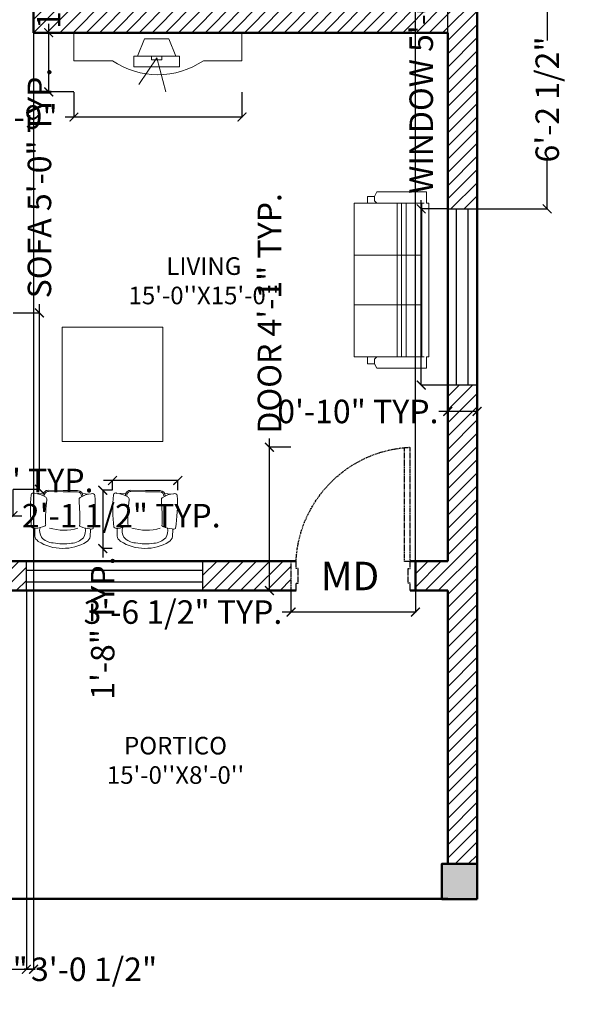
# Model space of a CAD drawing. Units: inches. Extents: x 1945 to 2401, y 1770 to 2289.
# Tile 4 of 5: x 2177 to 2369, y 1770 to 2105. Entities that reach past the tile are written whole.
import ezdxf

# ---------------------------------------------------------------- set-up
doc = ezdxf.new("R2010")
doc.units = ezdxf.units.IN
doc.linetypes.add('HIDDEN', pattern=[9.525, 6.35, -3.175])
for name, color, linetype, lineweight in [('A-ANNO-DIMS', 2, 'Continuous', 18), ('A-ANNO-TEXT', 7, 'Continuous', 18), ('A-AREA-IDEN', 7, 'Continuous', 25), ('A-COLS-PATT', 210, 'Continuous', 13), ('A-DOOR-HIDN', 150, 'HIDDEN', 25), ('A-WALL-PATT', 8, 'Continuous', 13), ('B-FURNITURE', 22, 'Continuous', 18), ('pillar', 210, 'Continuous', 50), ('Walls', 7, 'Continuous', 50), ('Windows', 32, 'Continuous', 25)]:
    doc.layers.add(name, color=color, linetype=linetype, lineweight=lineweight)
doc.styles.get("Standard").update_dxf_attribs({"font": 'arial.ttf'})
doc.dimstyles.get("Standard").update_dxf_attribs({"dimtxt": 8, "dimasz": 3, "dimexe": 0.18, "dimexo": 0.0625, "dimgap": 0.09, "dimtad": 0, "dimdec": 1, "dimzin": 0, "dimdsep": 46, "dimlunit": 4, "dimtxsty": 'Standard', "dimblk": 'ARCHTICK', "dimcen": 0.09, "dimadec": 0, "dimazin": 0, "dimtfac": 1, "dimtdec": 1, "dimtofl": 0, "dimtmove": 0, "dimatfit": 3, "dimfxl": 1, "dimtolj": 1, "dimtzin": 0, "dimarcsym": 0})

# ---------------------------------------------------------------- blocks, each defined once
blk = doc.blocks.new('A$C198557BC')
at = {"layer": 'B-FURNITURE'}
for p, q in [((-0.412, 0.581), (-0.41, 0.695)), ((0.425, 0.571), (0.425, 0.685)), ((-0.291, 0.046), (-0.382, 0.055)), ((-0.299, 0.083), (-0.299, 0.085)), ((0, 0.02), (-0.22, 0.023)), ((0, 0), (-0.22, 0.003)), ((0, 0.02), (0.221, 0.017)), ((0, 0), (0.22, -0.003)), ((0.291, 0.039), (0.383, 0.046)), ((0.301, 0.077), (0.301, 0.078))]:
    blk.add_line(p, q, dxfattribs=at)
for centre, radius, start, end in [((-0.288, 0.668), 0.124, 121.5636, 167.5307), ((-0.003, 0.196), 0.675, 88.9141, 121.2698), ((-0.109, 0.514), 0.28, 94.1154, 135.1368), ((-0.012, 0.135), 0.669, 87.9714, 100.088), ((0.005, 0.189), 0.683, 57.6049, 89.6023), ((-0.041, -0.271), 1.076, 79.8996, 87.1923), ((0.131, 0.526), 0.263, 42.8435, 86.2186), ((0.304, 0.661), 0.124, 11.1649, 57.132), ((-0.132, 0.606), 0.205, 148.9368, 191.7767), ((-0.015, -0.198), 0.795, 73.9397, 105.2329), ((0.146, 0.603), 0.205, 346.9189, 29.7588), ((1.987, 0.194), 2.469, 171.2505, 182.7738), ((-0.42, 0.533), 0.0491, 69.3538, 131.4415), ((-0.498, -0.067), 0.653, 68.9876, 81.6584), ((-0.269, 0.522), 0.0208, 332.4461, 75.1743), ((3.087, 0.412), 3.339, 178.2785, 184.601), ((-3.076, 0.483), 3.339, 354.0946, 0.4171), ((0.281, 0.516), 0.0208, 103.5213, 206.2495), ((0.496, -0.078), 0.653, 97.0372, 109.708), ((0.427, 0.504), 0.0668, 46.1176, 99.1612), ((-1.903, 0.273), 2.393, 354.9918, 6.6966), ((-0.444, 0.084), 0.0362, 194.4565, 300.6699), ((-0.452, 0.425), 0.374, 274.1336, 300.8386), ((-0.219, 0.083), 0.08, 179.3478, 269.3478), ((-0.219, 0.083), 0.06, 179.3478, 269.3478), ((-0.281, 0.139), 0.0403, 300.8178, 7.8066), ((0.221, 0.077), 0.08, 269.3478, 359.3478), ((0.221, 0.077), 0.06, 269.3478, 359.3478), ((0.284, 0.133), 0.0403, 170.889, 237.8778), ((0.462, 0.415), 0.374, 237.857, 264.562), ((0.446, 0.074), 0.0362, 238.0257, 344.2391)]:
    blk.add_arc(centre, radius, start, end, dxfattribs=at)
blk = doc.blocks.new('banghe81')
for p, q in [((-500, 3000), (0, 3000)), ((-500, 2312), (-500, 3000)), ((0, 3000), (0, 0)), ((-925, 1843), (-450, 1517)), ((-607, 1930), (-419, 1930)), ((-607, 1117), (-607, 1930)), ((-419, 1930), (-419, 1117)), ((-107, 1742), (-419, 1867)), ((-482, 1617), (-482, 1430)), ((-419, 1617), (-482, 1617)), ((-107, 1305), (-107, 1742)), ((-450, 1517), (-1057, 1361)), ((-482, 1430), (-419, 1430)), ((-419, 1180), (-107, 1305)), ((-419, 1117), (-607, 1117)), ((-500, 0), (-500, 688)), ((0, 0), (-500, 0)), ((-500, 0), (-500, 0))]:
    blk.add_line(p, q)
blk.add_arc((695, 1500), 1445, 145.7945, 214.2055)
blk = doc.blocks.new('12PCOU13')
at = {"color": 0, "linetype": 'ByBlock'}
for p, q in [((24, 35), (23, 34)), ((24, 37), (24, 35)), ((23, 34), (2, 34)), ((3, -34), (3, 34)), ((10, 34), (10, -34)), ((12, 34), (12, -34)), ((14, 34), (14, -34)), ((27, 34), (23, 34)), ((33, 11), (3, 11)), ((33, -11), (3, -11)), ((23, -34), (2, -34)), ((27, -34), (23, -34)), ((24, -35), (23, -34)), ((24, -37), (24, -35))]:
    blk.add_line(p, q, dxfattribs=at)
blk.add_lwpolyline([(1, -39), (1, -34), (0, -34), (0, 34), (1, 34), (1, 39), (23, 39), (24, 37), (27, 37), (27, 34), (33, 34), (33, -34), (27, -34), (27, -37), (24, -37), (23, -39)], close=True, dxfattribs=at)
blk = doc.blocks.new('AP0B05')
for p, q in [((35, 100), (35, 880)), ((75, 100), (75, 878.9))]:
    blk.add_line(p, q)
for points in [[(0, 100), (0, -100), (35, -100), (35, -50), (50, -50), (50, 50), (35, 50), (35, 100)], [(850, 100), (850, -100), (815, -100), (815, -50), (800, -50), (800, 50), (815, 50), (815, 100)]]:
    blk.add_lwpolyline(points, close=True)
blk.add_lwpolyline([(35, 100), (75, 100)])
blk.add_arc((-2.4, 62.6), 818.3, 2.62122, 87.37878)
blk = doc.blocks.new('WIN-60IN')
for p, q in [((0, 7), (60, 7)), ((0, 3), (60, 3))]:
    blk.add_line(p, q)
blk.add_lwpolyline([(0, 10), (60, 10), (60, 0), (0, 0)], close=True)
blk = doc.blocks.new('_ArchTick')
at = {"color": 0, "linetype": 'ByBlock', "const_width": 0.15}
blk.add_lwpolyline([(-0.5, -0.5), (0.5, 0.5)], dxfattribs=at)
blk = doc.blocks.new('*D33')
at = {"layer": 'A-ANNO-DIMS', "color": 0, "lineweight": -2, "transparency": 16777216}
for p, q in [((2262.17, 1959.86), (2262.17, 1962.86)), ((2269.43, 1959.86), (2261.99, 1959.86)), ((2262.17, 1911.04), (2262.17, 1959.86)), ((2269.43, 1911.04), (2261.99, 1911.04))]:
    blk.add_line(p, q, dxfattribs=at)
at = {"layer": 'Defpoints', "color": 0, "transparency": 16777216}
for p in [(2262.17, 1959.86), (2269.5, 1959.86), (2269.5, 1911.04)]:
    blk.add_point(p, dxfattribs=at)
at = {"layer": 'A-ANNO-DIMS', "color": 0, "lineweight": -2, "transparency": 16777216, "xscale": 3, "yscale": 3, "zscale": 3}
for p, rotation in [((2262.17, 1959.86), 90), ((2262.17, 1911.04), 270)]:
    blk.add_blockref('_ArchTick', p, dxfattribs=dict(at, rotation=rotation))
at = {"layer": 'A-ANNO-DIMS', "color": 0, "transparency": 16777216, "insert": (2262.17, 2005.45), "char_height": 8, "attachment_point": 5, "rotation": 90}
blk.add_mtext('\\A1;DOOR 4\'-1" TYP.', dxfattribs=at)
blk = doc.blocks.new('*D34')
at = {"layer": 'A-ANNO-DIMS', "color": 0, "lineweight": -2, "transparency": 16777216}
for p, q in [((2269.5, 1910.98), (2269.5, 1903.54)), ((2311.84, 1910.98), (2311.84, 1903.54)), ((2269.5, 1903.72), (2266.5, 1903.72)), ((2311.84, 1903.72), (2269.5, 1903.72))]:
    blk.add_line(p, q, dxfattribs=at)
at = {"layer": 'Defpoints', "color": 0, "transparency": 16777216}
for p in [(2269.5, 1911.04), (2311.84, 1911.04), (2269.5, 1903.72)]:
    blk.add_point(p, dxfattribs=at)
at = {"layer": 'A-ANNO-DIMS', "color": 0, "lineweight": -2, "transparency": 16777216, "xscale": 3, "yscale": 3, "zscale": 3, "rotation": 180}
blk.add_blockref('_ArchTick', (2269.5, 1903.72), dxfattribs=at)
at = {"layer": 'A-ANNO-DIMS', "color": 0, "lineweight": -2, "transparency": 16777216, "xscale": 3, "yscale": 3, "zscale": 3}
blk.add_blockref('_ArchTick', (2311.84, 1903.72), dxfattribs=at)
at = {"layer": 'A-ANNO-DIMS', "color": 0, "transparency": 16777216, "insert": (2232.71, 1903.72), "char_height": 8, "attachment_point": 5}
blk.add_mtext('\\A1;3\'-6 1/2" TYP.', dxfattribs=at)
blk = doc.blocks.new('*D35')
at = {"layer": 'A-ANNO-DIMS', "color": 0, "lineweight": -2, "transparency": 16777216}
for p, q in [((2313.84, 2041.04), (2313.84, 2044.04)), ((2322.78, 2041.04), (2313.66, 2041.04)), ((2313.84, 1981.04), (2313.84, 2041.04)), ((2322.78, 1981.04), (2313.66, 1981.04))]:
    blk.add_line(p, q, dxfattribs=at)
at = {"layer": 'Defpoints', "color": 0, "transparency": 16777216}
for p in [(2313.84, 2041.04), (2322.84, 2041.04), (2322.84, 1981.04)]:
    blk.add_point(p, dxfattribs=at)
at = {"layer": 'A-ANNO-DIMS', "color": 0, "lineweight": -2, "transparency": 16777216, "xscale": 3, "yscale": 3, "zscale": 3}
for p, rotation in [((2313.84, 2041.04), 90), ((2313.84, 1981.04), 270)]:
    blk.add_blockref('_ArchTick', p, dxfattribs=dict(at, rotation=rotation))
at = {"layer": 'A-ANNO-DIMS', "color": 0, "transparency": 16777216, "insert": (2313.84, 2094.75), "char_height": 8, "attachment_point": 5, "rotation": 90}
blk.add_mtext('\\A1;WINDOW 5\'-0" TYP.', dxfattribs=at)
blk = doc.blocks.new('*D36')
at = {"layer": 'A-ANNO-DIMS', "color": 0, "lineweight": -2, "transparency": 16777216}
for p, q in [((2322.84, 1980.98), (2322.84, 1971.86)), ((2332.84, 1980.98), (2332.84, 1971.86)), ((2322.84, 1972.04), (2319.84, 1972.04)), ((2332.84, 1972.04), (2322.84, 1972.04))]:
    blk.add_line(p, q, dxfattribs=at)
at = {"layer": 'Defpoints', "color": 0, "transparency": 16777216}
for p in [(2322.84, 1981.04), (2332.84, 1981.04), (2322.84, 1972.04)]:
    blk.add_point(p, dxfattribs=at)
at = {"layer": 'A-ANNO-DIMS', "color": 0, "lineweight": -2, "transparency": 16777216, "xscale": 3, "yscale": 3, "zscale": 3, "rotation": 180}
blk.add_blockref('_ArchTick', (2322.84, 1972.04), dxfattribs=at)
at = {"layer": 'A-ANNO-DIMS', "color": 0, "lineweight": -2, "transparency": 16777216, "xscale": 3, "yscale": 3, "zscale": 3}
blk.add_blockref('_ArchTick', (2332.84, 1972.04), dxfattribs=at)
at = {"layer": 'A-ANNO-DIMS', "color": 0, "transparency": 16777216, "insert": (2292.26, 1972.04), "char_height": 8, "attachment_point": 5}
blk.add_mtext('\\A1;0\'-10" TYP.', dxfattribs=at)
blk = doc.blocks.new('*D37')
at = {"layer": 'A-ANNO-DIMS', "color": 0, "lineweight": -2, "transparency": 16777216}
for p, q in [((2183.86, 2005.62), (2183.86, 2008.62)), ((2174.92, 2005.62), (2184.04, 2005.62)), ((2183.86, 1945.56), (2183.86, 2005.62)), ((2174.92, 1945.56), (2184.04, 1945.56))]:
    blk.add_line(p, q, dxfattribs=at)
at = {"layer": 'Defpoints', "color": 0, "transparency": 16777216}
for p in [(2174.85, 2005.62), (2183.86, 2005.62), (2174.85, 1945.56)]:
    blk.add_point(p, dxfattribs=at)
at = {"layer": 'A-ANNO-DIMS', "color": 0, "lineweight": -2, "transparency": 16777216, "xscale": 3, "yscale": 3, "zscale": 3}
for p, rotation in [((2183.86, 2005.62), 90), ((2183.86, 1945.56), 270)]:
    blk.add_blockref('_ArchTick', p, dxfattribs=dict(at, rotation=rotation))
at = {"layer": 'A-ANNO-DIMS', "color": 0, "transparency": 16777216, "insert": (2183.86, 2049.84), "char_height": 8, "attachment_point": 5, "rotation": 90}
blk.add_mtext('\\A1;SOFA 5\'-0" TYP.', dxfattribs=at)
blk = doc.blocks.new('*D38')
at = {"layer": 'A-ANNO-DIMS', "color": 0, "lineweight": -2, "transparency": 16777216}
for p, q in [((2149.44, 1945.5), (2149.44, 1936.37)), ((2174.85, 1945.5), (2174.85, 1936.37)), ((2149.44, 1936.55), (2174.85, 1936.55)), ((2174.85, 1936.55), (2177.85, 1936.55))]:
    blk.add_line(p, q, dxfattribs=at)
at = {"layer": 'Defpoints', "color": 0, "transparency": 16777216}
for p in [(2149.44, 1945.56), (2174.85, 1945.56), (2174.85, 1936.55)]:
    blk.add_point(p, dxfattribs=at)
at = {"layer": 'A-ANNO-DIMS', "color": 0, "lineweight": -2, "transparency": 16777216, "xscale": 3, "yscale": 3, "zscale": 3, "rotation": 180}
blk.add_blockref('_ArchTick', (2149.44, 1936.55), dxfattribs=at)
at = {"layer": 'A-ANNO-DIMS', "color": 0, "lineweight": -2, "transparency": 16777216, "xscale": 3, "yscale": 3, "zscale": 3}
blk.add_blockref('_ArchTick', (2174.85, 1936.55), dxfattribs=at)
at = {"layer": 'A-ANNO-DIMS', "color": 0, "transparency": 16777216, "insert": (2211.71, 1936.55), "char_height": 8, "attachment_point": 5}
blk.add_mtext('\\A1;2\'-1 1/2" TYP.', dxfattribs=at)
blk = doc.blocks.new('*D39')
at = {"layer": 'A-ANNO-DIMS', "color": 0, "lineweight": -2, "transparency": 16777216}
for p, q in [((2208.72, 1948.53), (2205.72, 1948.53)), ((2208.72, 1945.26), (2208.72, 1948.71)), ((2230.95, 1948.53), (2208.72, 1948.53)), ((2230.95, 1945.26), (2230.95, 1948.71))]:
    blk.add_line(p, q, dxfattribs=at)
at = {"layer": 'Defpoints', "color": 0, "transparency": 16777216}
for p in [(2208.72, 1948.53), (2208.72, 1945.2), (2230.95, 1945.2)]:
    blk.add_point(p, dxfattribs=at)
at = {"layer": 'A-ANNO-DIMS', "color": 0, "lineweight": -2, "transparency": 16777216, "xscale": 3, "yscale": 3, "zscale": 3, "rotation": 180}
blk.add_blockref('_ArchTick', (2208.72, 1948.53), dxfattribs=at)
at = {"layer": 'A-ANNO-DIMS', "color": 0, "lineweight": -2, "transparency": 16777216, "xscale": 3, "yscale": 3, "zscale": 3}
blk.add_blockref('_ArchTick', (2230.95, 1948.53), dxfattribs=at)
at = {"layer": 'A-ANNO-DIMS', "color": 0, "transparency": 16777216, "insert": (2146.55, 1948.53), "char_height": 8, "attachment_point": 5}
blk.add_mtext('\\A1;ARMCHAIR 1\'-10" TYP.', dxfattribs=at)
blk = doc.blocks.new('*D40')
at = {"layer": 'A-ANNO-DIMS', "color": 0, "lineweight": -2, "transparency": 16777216}
for p, q in [((2208.66, 1945.2), (2205.21, 1945.2)), ((2205.39, 1945.2), (2205.39, 1925.34)), ((2208.66, 1925.34), (2205.21, 1925.34)), ((2205.39, 1925.34), (2205.39, 1922.34))]:
    blk.add_line(p, q, dxfattribs=at)
at = {"layer": 'Defpoints', "color": 0, "transparency": 16777216}
for p in [(2208.72, 1945.2), (2205.39, 1925.34), (2208.72, 1925.34)]:
    blk.add_point(p, dxfattribs=at)
at = {"layer": 'A-ANNO-DIMS', "color": 0, "lineweight": -2, "transparency": 16777216, "xscale": 3, "yscale": 3, "zscale": 3}
for p, rotation in [((2205.39, 1945.2), 90), ((2205.39, 1925.34), 270)]:
    blk.add_blockref('_ArchTick', p, dxfattribs=dict(at, rotation=rotation))
at = {"layer": 'A-ANNO-DIMS', "color": 0, "transparency": 16777216, "insert": (2205.39, 1898.25), "char_height": 8, "attachment_point": 5, "rotation": 90}
blk.add_mtext('\\A1;1\'-8" TYP.', dxfattribs=at)
blk = doc.blocks.new('*D55')
at = {"layer": 'A-ANNO-DIMS', "color": 0, "lineweight": -2, "transparency": 16777216}
for p, q in [((2195.59, 2080.82), (2195.59, 2072.12)), ((2252.8, 2080.82), (2252.8, 2072.12)), ((2195.59, 2072.3), (2192.59, 2072.3)), ((2252.8, 2072.3), (2195.59, 2072.3))]:
    blk.add_line(p, q, dxfattribs=at)
at = {"layer": 'Defpoints', "color": 0, "transparency": 16777216}
for p in [(2195.59, 2080.88), (2252.8, 2080.88), (2195.59, 2072.3)]:
    blk.add_point(p, dxfattribs=at)
at = {"layer": 'A-ANNO-DIMS', "color": 0, "lineweight": -2, "transparency": 16777216, "xscale": 3, "yscale": 3, "zscale": 3, "rotation": 180}
blk.add_blockref('_ArchTick', (2195.59, 2072.3), dxfattribs=at)
at = {"layer": 'A-ANNO-DIMS', "color": 0, "lineweight": -2, "transparency": 16777216, "xscale": 3, "yscale": 3, "zscale": 3}
blk.add_blockref('_ArchTick', (2252.8, 2072.3), dxfattribs=at)
at = {"layer": 'A-ANNO-DIMS', "color": 0, "transparency": 16777216, "insert": (2144.19, 2072.3), "char_height": 8, "attachment_point": 5}
blk.add_mtext('\\A1;TV CONSOLE 4\'-9"', dxfattribs=at)
blk = doc.blocks.new('*D56')
at = {"layer": 'A-ANNO-DIMS', "color": 0, "lineweight": -2, "transparency": 16777216}
for p, q in [((2187, 2101.04), (2187, 2104.04)), ((2195.52, 2101.04), (2186.82, 2101.04)), ((2187, 2080.88), (2187, 2101.04)), ((2195.52, 2080.88), (2186.82, 2080.88))]:
    blk.add_line(p, q, dxfattribs=at)
at = {"layer": 'Defpoints', "color": 0, "transparency": 16777216}
for p in [(2187, 2101.04), (2195.59, 2101.04), (2195.59, 2080.88)]:
    blk.add_point(p, dxfattribs=at)
at = {"layer": 'A-ANNO-DIMS', "color": 0, "lineweight": -2, "transparency": 16777216, "xscale": 3, "yscale": 3, "zscale": 3}
for p, rotation in [((2187, 2101.04), 90), ((2187, 2080.88), 270)]:
    blk.add_blockref('_ArchTick', p, dxfattribs=dict(at, rotation=rotation))
at = {"layer": 'A-ANNO-DIMS', "color": 0, "transparency": 16777216, "insert": (2187, 2114.39), "char_height": 8, "attachment_point": 5, "rotation": 90}
blk.add_mtext('\\A1;1\'-8"', dxfattribs=at)
blk = doc.blocks.new('*D61')
at = {"layer": 'A-ANNO-DIMS', "color": 0, "lineweight": -2, "transparency": 16777216}
for p, q in [((2332.9, 2115.57), (2356.92, 2115.57)), ((2356.74, 2115.57), (2356.74, 2098.37)), ((2356.74, 2041.04), (2356.74, 2058.24)), ((2332.9, 2041.04), (2356.92, 2041.04))]:
    blk.add_line(p, q, dxfattribs=at)
at = {"layer": 'Defpoints', "color": 0, "transparency": 16777216}
for p in [(2332.84, 2115.57), (2332.84, 2041.04), (2356.74, 2041.04)]:
    blk.add_point(p, dxfattribs=at)
at = {"layer": 'A-ANNO-DIMS', "color": 0, "lineweight": -2, "transparency": 16777216, "xscale": 3, "yscale": 3, "zscale": 3}
for p, rotation in [((2356.74, 2115.57), 90), ((2356.74, 2041.04), 270)]:
    blk.add_blockref('_ArchTick', p, dxfattribs=dict(at, rotation=rotation))
at = {"layer": 'A-ANNO-DIMS', "color": 0, "transparency": 16777216, "insert": (2356.74, 2078.3), "char_height": 8, "attachment_point": 5, "rotation": 90}
blk.add_mtext('\\A1;6\'-2 1/2"', dxfattribs=at)
blk = doc.blocks.new('*D65')
at = {"layer": 'A-ANNO-DIMS', "color": 0, "lineweight": -2, "transparency": 16777216}
for p, q in [((2142.84, 1910.98), (2142.84, 1781.89)), ((2179.42, 1910.98), (2179.42, 1781.89)), ((2142.84, 1782.07), (2179.42, 1782.07)), ((2179.42, 1782.07), (2182.42, 1782.07))]:
    blk.add_line(p, q, dxfattribs=at)
at = {"layer": 'Defpoints', "color": 0, "transparency": 16777216}
for p in [(2142.84, 1911.04), (2179.42, 1911.04), (2179.42, 1782.07)]:
    blk.add_point(p, dxfattribs=at)
at = {"layer": 'A-ANNO-DIMS', "color": 0, "lineweight": -2, "transparency": 16777216, "xscale": 3, "yscale": 3, "zscale": 3, "rotation": 180}
blk.add_blockref('_ArchTick', (2142.84, 1782.07), dxfattribs=at)
at = {"layer": 'A-ANNO-DIMS', "color": 0, "lineweight": -2, "transparency": 16777216, "xscale": 3, "yscale": 3, "zscale": 3}
blk.add_blockref('_ArchTick', (2179.42, 1782.07), dxfattribs=at)
at = {"layer": 'A-ANNO-DIMS', "color": 0, "transparency": 16777216, "insert": (2202.46, 1782.07), "char_height": 8, "attachment_point": 5}
blk.add_mtext('\\A1;3\'-0 1/2"', dxfattribs=at)
blk = doc.blocks.new('*D66')
at = {"layer": 'A-ANNO-DIMS', "color": 0, "lineweight": -2, "transparency": 16777216}
for p, q in [((2311.84, 1921.1), (2311.84, 2277.12)), ((2311.84, 2276.94), (2322.84, 2276.94)), ((2322.84, 1921.1), (2322.84, 2277.12)), ((2322.84, 2276.94), (2325.84, 2276.94))]:
    blk.add_line(p, q, dxfattribs=at)
at = {"layer": 'Defpoints', "color": 0, "transparency": 16777216}
for p in [(2322.84, 2276.94), (2311.84, 1921.04), (2322.84, 1921.04)]:
    blk.add_point(p, dxfattribs=at)
at = {"layer": 'A-ANNO-DIMS', "color": 0, "lineweight": -2, "transparency": 16777216, "xscale": 3, "yscale": 3, "zscale": 3, "rotation": 180}
blk.add_blockref('_ArchTick', (2311.84, 2276.94), dxfattribs=at)
at = {"layer": 'A-ANNO-DIMS', "color": 0, "lineweight": -2, "transparency": 16777216, "xscale": 3, "yscale": 3, "zscale": 3}
blk.add_blockref('_ArchTick', (2322.84, 2276.94), dxfattribs=at)
at = {"layer": 'A-ANNO-DIMS', "color": 0, "transparency": 16777216, "insert": (2339.67, 2276.94), "char_height": 8, "attachment_point": 5}
blk.add_mtext('\\A1;0\'-11"', dxfattribs=at)
blk = doc.blocks.new('*D70')
at = {"layer": 'A-ANNO-DIMS', "color": 0, "lineweight": -2, "transparency": 16777216}
for p, q in [((2153.84, 2100.98), (2153.84, 1781.89)), ((2181.84, 2100.98), (2181.84, 1781.89)), ((2153.84, 1782.07), (2157.05, 1782.07)), ((2181.84, 1782.07), (2178.63, 1782.07))]:
    blk.add_line(p, q, dxfattribs=at)
at = {"layer": 'Defpoints', "color": 0, "transparency": 16777216}
for p in [(2153.84, 2101.04), (2181.84, 2101.04), (2181.84, 1782.07)]:
    blk.add_point(p, dxfattribs=at)
at = {"layer": 'A-ANNO-DIMS', "color": 0, "lineweight": -2, "transparency": 16777216, "xscale": 3, "yscale": 3, "zscale": 3, "rotation": 180}
blk.add_blockref('_ArchTick', (2153.84, 1782.07), dxfattribs=at)
at = {"layer": 'A-ANNO-DIMS', "color": 0, "lineweight": -2, "transparency": 16777216, "xscale": 3, "yscale": 3, "zscale": 3}
blk.add_blockref('_ArchTick', (2181.84, 1782.07), dxfattribs=at)
at = {"layer": 'A-ANNO-DIMS', "color": 0, "transparency": 16777216, "insert": (2167.84, 1782.07), "char_height": 8, "attachment_point": 5}
blk.add_mtext('\\A1;2\'-4"', dxfattribs=at)

msp = doc.modelspace()

# ---------------------------------------------------------------- hatches: boundary and pattern name
at = {"layer": 'A-COLS-PATT'}
h = msp.add_hatch(color=256, dxfattribs=at)
h.dxf.hatch_style = 1
h.paths.add_polyline_path([(2332.84, 1817.97), (2320.84, 1817.97), (2320.84, 1806.04), (2322.84, 1806.04), (2332.84, 1805.97)])
at = {"layer": 'A-WALL-PATT', "transparency": 33554585}
h = msp.add_hatch(dxfattribs=at)
h.set_pattern_fill('ANSI31', color=256)
h.paths.add_polyline_path([(2151.34, 2253.04), (2002.84, 2253.04), (2002.84, 2158.54), (2012.84, 2158.54), (2012.84, 2243.04), (2132.84, 2243.04), (2132.88, 2160.39), (2142.84, 2160.39), (2142.84, 2165.04), (2192.84, 2165.04), (2192.84, 2160.39), (2202.84, 2160.39), (2202.84, 2175.04), (2192.84, 2175.04), (2192.84, 2171.04), (2138.84, 2171.04), (2138.84, 2243.04), (2151.34, 2243.04)])
h.paths.add_polyline_path([(2332.84, 2253.04), (2180.34, 2253.04), (2180.34, 2243.04), (2192.84, 2243.04), (2192.84, 2207.47), (2202.84, 2207.47), (2202.84, 2243.04), (2322.84, 2243.04), (2322.84, 2175.57), (2332.84, 2175.57)])
h.paths.add_polyline_path([(2012.84, 2105.04), (2041.41, 2105.04), (2041.41, 2111.04), (2012.84, 2111.04), (2012.84, 2122.54), (2002.84, 2122.54), (2002.84, 2055.45), (2012.84, 2055.45)])
h.paths.add_polyline_path([(2332.84, 2115.57), (2322.84, 2115.57), (2322.84, 2111.04), (2202.84, 2111.04), (2202.84, 2118.04), (2192.84, 2118.04), (2192.84, 2111.04), (2181.84, 2111.04), (2181.84, 2101.04), (2322.84, 2101.04), (2322.84, 2041.04), (2332.84, 2041.04)])
h = msp.add_hatch(dxfattribs=at)
h.set_pattern_fill('ANSI31', color=256)
h.paths.add_polyline_path([(2142.84, 2006.04), (2132.84, 2006.04), (2132.84, 1898.04), (2012.84, 1898.04), (2012.84, 1888.04), (2142.84, 1888.04), (2142.84, 1911.04), (2179.42, 1911.04), (2179.42, 1921.04), (2142.84, 1921.04)])
h.paths.add_polyline_path([(2269.5, 1921.04), (2239.42, 1921.04), (2239.42, 1911.04), (2269.5, 1911.04)])
h.paths.add_polyline_path([(2332.84, 1981.04), (2322.84, 1981.04), (2322.84, 1921.04), (2311.84, 1921.04), (2311.84, 1911.04), (2322.84, 1911.04), (2322.84, 1817.97), (2332.84, 1817.97)])
h.paths.add_polyline_path([(2012.84, 1931.04), (2002.84, 1931.04), (2002.84, 1806.04), (2142.84, 1806.04), (2142.84, 1816.04), (2012.84, 1816.04)])
h.paths.add_polyline_path([(2012.84, 2000.04), (2082.92, 2000.04), (2082.92, 2006.04), (2066.84, 2006.04), (2066.84, 2101.04), (2142.84, 2101.04), (2153.84, 2101.04), (2153.84, 2111.04), (2142.84, 2111.04), (2142.84, 2118.04), (2132.84, 2118.04), (2132.84, 2111.04), (2060.84, 2111.04), (2060.84, 2006.04), (2012.84, 2006.04), (2012.84, 2026.45), (2002.84, 2026.45), (2002.84, 1967.04), (2012.84, 1967.04)])

# ---------------------------------------------------------------- linework, layer by layer
at = {"layer": 'B-FURNITURE'}
msp.add_lwpolyline([(2191.6, 2000.7), (2225.87, 2000.7), (2225.87, 1961.83), (2191.6, 1961.83)], close=True, dxfattribs=at)
at = {"layer": 'pillar'}
msp.add_lwpolyline([(2332.84, 1805.97), (2320.84, 1805.97), (2320.84, 1817.97), (2332.84, 1817.97)], close=True, dxfattribs=at)
at = {"layer": 'Walls'}
for p, q in [((2332.84, 2253.04), (2332.84, 1805.97)), ((2181.84, 2111.04), (2181.84, 2101.04)), ((2181.84, 2101.04), (2322.84, 2101.04)), ((2322.84, 2101.04), (2322.84, 1921.04)), ((2142.84, 1921.04), (2271.24, 1921.04)), ((2310.1, 1921.04), (2322.84, 1921.04)), ((2311.84, 1921.04), (2311.84, 1911.04)), ((2142.84, 1911.04), (2271.24, 1911.04)), ((2310.1, 1911.04), (2322.84, 1911.04)), ((2322.84, 1911.04), (2322.84, 1817.97)), ((2002.84, 1806.04), (2322.84, 1806.04)), ((2322.84, 1806.04), (2322.84, 1805.97))]:
    msp.add_line(p, q, dxfattribs=at)

# ---------------------------------------------------------------- block references
at = {"layer": 'A-DOOR-HIDN', "xscale": -0.0498193668704145, "yscale": 0.0498193668704145, "zscale": 0.0498193668704145}
msp.add_blockref('AP0B05', (2311.84, 1916.02), dxfattribs=at)
at = {"layer": 'B-FURNITURE'}
for name, p, xscale, yscale, zscale, rotation in [('banghe81', (2252.8, 2101.04), 0.0190699229775345, 0.0190699229775345, 0.0190699229775345, 90), ('12PCOU13', (2316.39, 2016.81), 0.770001005946072, 0.770001005946072, 0.770001005946072, 180), ('A$C198557BC', (2191.88, 1945.14), 22.64915604914234, 22.64915604914234, 22.64915604914234, 180), ('A$C198557BC', (2219.92, 1945.14), 22.64915604914234, 22.64915604914234, 22.64915604914234, 180)]:
    msp.add_blockref(name, p, dxfattribs=dict(at, xscale=xscale, yscale=yscale, zscale=zscale, rotation=rotation))
at = {"layer": 'Windows', "rotation": 89.99999999999962}
msp.add_blockref('WIN-60IN', (2332.84, 1981.04), dxfattribs=at)
at = {"layer": 'Windows'}
msp.add_blockref('WIN-60IN', (2179.42, 1911.04), dxfattribs=at)

# ---------------------------------------------------------------- texts
at = {"layer": 'A-ANNO-TEXT'}
msp.add_text('MD', height=9.712, dxfattribs=at).set_placement((2279.66, 1911.15))
at = {"layer": 'A-AREA-IDEN', "char_height": 6, "attachment_point": 1}
for s, insert in [("\\pxqc;LIVING\\P15'-0''X15'-0''", (2213.66, 2024.55)), ("\\pxqc;PORTICO\\P15'-0''X8'-0''", (2204.01, 1861.23))]:
    msp.add_mtext_dynamic_manual_height_columns(s, width=52.3454, gutter_width=12.5, heights=[0], dxfattribs=dict(at, insert=insert))

# ---------------------------------------------------------------- dimensions: what is measured, and where the dimension line sits
at = {"layer": 'A-ANNO-DIMS'}
for base, p1, p2, picture, middle in [((2322.84, 2276.94), (2311.84, 1921.04), (2322.84, 1921.04), '*D66', (2339.67, 2276.94)), ((2181.84, 1782.07), (2153.84, 2101.04), (2181.84, 2101.04), '*D70', (2167.84, 1782.07)), ((2179.42, 1782.07), (2142.84, 1911.04), (2179.42, 1911.04), '*D65', (2202.46, 1782.07))]:
    dim = msp.add_linear_dim(base=base, p1=p1, p2=p2, dimstyle='Standard', override={"dimdec": 1, "dimlfac": 1, "dimrnd": 0, "dimzin": 1, "dimdsep": 46, "dimlunit": 4, "dimfrac": 2}, dxfattribs=at)
    dim.commit()
    dim.dimension.update_dxf_attribs({"geometry": picture, "text_midpoint": middle})
for base, p1, p2, angle, text, picture, middle in [((2313.84, 2041.04), (2322.84, 1981.04), (2322.84, 2041.04), 90, 'WINDOW <> TYP.', '*D35', (2313.84, 2094.75)), ((2195.59, 2072.3), (2252.8, 2080.88), (2195.59, 2080.88), 180, 'TV CONSOLE <>', '*D55', (2144.19, 2072.3)), ((2183.86, 2005.62), (2174.85, 1945.56), (2174.85, 2005.62), 90, 'SOFA <> TYP.', '*D37', (2183.86, 2049.84)), ((2262.17, 1959.86), (2269.5, 1911.04), (2269.5, 1959.86), 90, 'DOOR <> TYP.', '*D33', (2262.17, 2005.45)), ((2322.84, 1972.04), (2332.84, 1981.04), (2322.84, 1981.04), 180, '<> TYP.', '*D36', (2292.26, 1972.04)), ((2208.72, 1948.53), (2230.95, 1945.2), (2208.72, 1945.2), 180, 'ARMCHAIR <> TYP.', '*D39', (2146.55, 1948.53)), ((2205.39, 1925.34), (2208.72, 1945.2), (2208.72, 1925.34), 270, '<> TYP.', '*D40', (2205.39, 1898.25)), ((2269.5, 1903.72), (2311.84, 1911.04), (2269.5, 1911.04), 180, '<> TYP.', '*D34', (2232.71, 1903.72))]:
    dim = msp.add_linear_dim(base=base, p1=p1, p2=p2, angle=angle, text=text, dimstyle='Standard', override={"dimdec": 1, "dimlfac": 1, "dimrnd": 0, "dimzin": 1, "dimdsep": 46, "dimlunit": 4, "dimfrac": 2}, dxfattribs=at)
    dim.commit()
    dim.dimension.update_dxf_attribs({"geometry": picture, "text_midpoint": middle})
for base, p1, p2, picture, middle in [((2187, 2101.04), (2195.59, 2080.88), (2195.59, 2101.04), '*D56', (2187, 2114.39)), ((2356.74, 2041.04), (2332.84, 2115.57), (2332.84, 2041.04), '*D61', (2356.74, 2078.3))]:
    dim = msp.add_linear_dim(base=base, p1=p1, p2=p2, angle=90, dimstyle='Standard', override={"dimdec": 1, "dimlfac": 1, "dimrnd": 0, "dimzin": 1, "dimdsep": 46, "dimlunit": 4, "dimfrac": 2}, dxfattribs=at)
    dim.commit()
    dim.dimension.update_dxf_attribs({"geometry": picture, "text_midpoint": middle})
dim = msp.add_linear_dim(base=(2174.85, 1936.55), p1=(2149.44, 1945.56), p2=(2174.85, 1945.56), text='<> TYP.', dimstyle='Standard', override={"dimdec": 1, "dimlfac": 1, "dimrnd": 0, "dimzin": 1, "dimdsep": 46, "dimlunit": 4, "dimfrac": 2}, dxfattribs=at)
dim.commit()
dim.dimension.update_dxf_attribs({"geometry": '*D38', "text_midpoint": (2211.71, 1936.55)})

doc.saveas('drawing.dxf')
